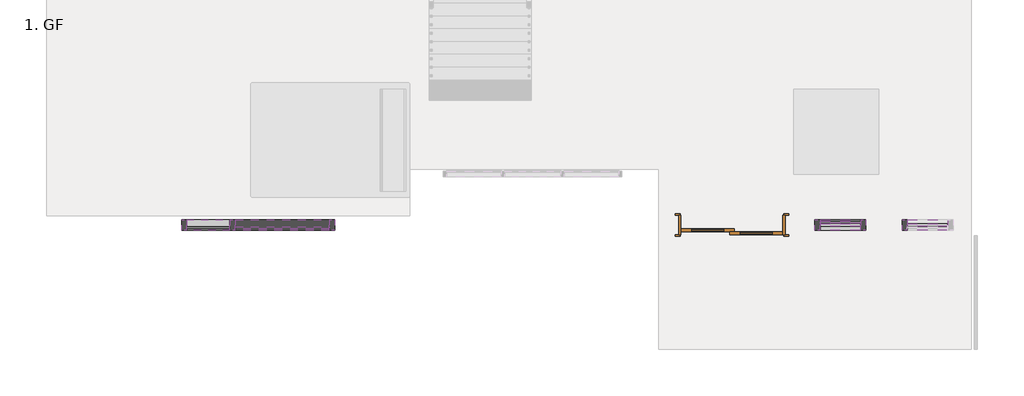
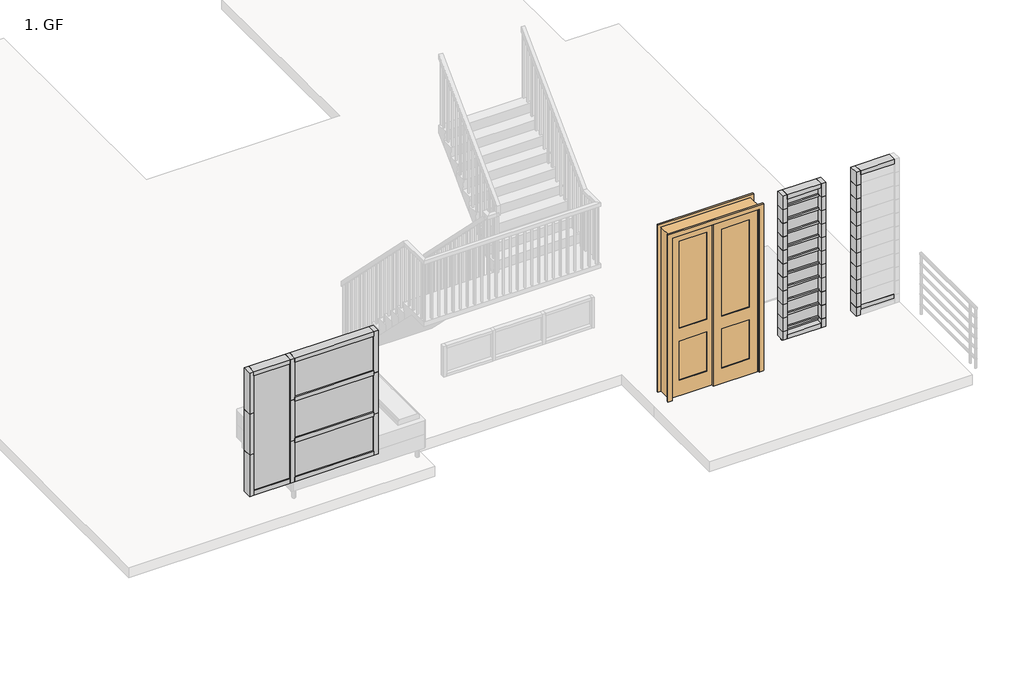
# One storey, part 1 of 3: 72 members, 16 plates, 1 door.
"""IFC4 building model written with IfcOpenShell, lengths in millimetres."""

from ifc_helpers import new_model, si_unit, origin, place, context, project, spatial, transform, mapped, element, save
from components import door_interior_double_sliding_2_panel_wood_4_x8_84ebb68c, member_93b5357b, member_3e1f1dd8, member_86d06fe4, member_a8054089, member_a8e3eee7, member_0b7646a3, member_e6b9f524, member_2cd1b1d9, member_866a01fa, member_c3a59c23, system_panel_glazed_ee894bee, system_panel_glazed_9eb8e914, system_panel_glazed_008e37cc, system_panel_glazed_06acdacc, system_panel_glazed_f6e37d5f, system_panel_glazed_d1e8daba

model = new_model("IFC4")

# Units and contexts
model_context = context("Model", 3, world=origin())
ifc_project = project(units=[si_unit("LENGTHUNIT", "METRE", prefix="MILLI")], contexts=[model_context])

# Site, building, storey
site = spatial("IfcSite", under=ifc_project)
building = spatial("IfcBuilding", under=site)
storey = spatial("IfcBuildingStorey", under=building, Name="1. GF", Elevation=609.6)

# Door
placement = place(None, origin())
door_interior_double_sliding_2_panel_wood_4_x8_shape = door_interior_double_sliding_2_panel_wood_4_x8_84ebb68c(model_context)
element("IfcDoor", 1, ObjectType="Door-Interior-Double-Sliding-2_Panel-Wood : 4' X8'", at=placement, inside=storey, context=model_context, shape_type="MappedRepresentation", body=[
    mapped(door_interior_double_sliding_2_panel_wood_4_x8_shape, transform((855.0250448, -610.2589711, 609.6), x_axis=(-1.0, 0.0, 0.0), y_axis=(0.0, -1.0, 0.0), z_axis=(0.0, 0.0, 1.0))),
])

# Members
member_shape = member_93b5357b(model_context)
element("IfcMember", 2, ObjectType="Rectangular Mullion : 1\" Square", at=placement, inside=storey, context=model_context, shape_type="MappedRepresentation", body=[
    mapped(member_shape, transform((2391.7250448, -607.0839711, 2463.8), x_axis=(0.0, 0.0, 1.0), y_axis=(0.0, -1.0, 0.0), z_axis=(1.0, 0.0, 0.0))),
])
element("IfcMember", 3, ObjectType="Rectangular Mullion : 1\" Square", at=placement, inside=storey, context=model_context, shape_type="MappedRepresentation", body=[
    mapped(member_shape, transform((2391.7250448, -607.0839711, 2667.0), x_axis=(0.0, 0.0, 1.0), y_axis=(0.0, -1.0, 0.0), z_axis=(1.0, 0.0, 0.0))),
])
element("IfcMember", 4, ObjectType="Rectangular Mullion : 1\" Square", at=placement, inside=storey, context=model_context, shape_type="MappedRepresentation", body=[
    mapped(member_shape, transform((2391.7250448, -607.0839711, 2260.6), x_axis=(0.0, 0.0, 1.0), y_axis=(0.0, -1.0, 0.0), z_axis=(1.0, 0.0, 0.0))),
])
element("IfcMember", 5, ObjectType="Rectangular Mullion : 1\" Square", at=placement, inside=storey, context=model_context, shape_type="MappedRepresentation", body=[
    mapped(member_shape, transform((2391.7250448, -607.0839711, 2057.4), x_axis=(0.0, 0.0, 1.0), y_axis=(0.0, -1.0, 0.0), z_axis=(1.0, 0.0, 0.0))),
])
element("IfcMember", 6, ObjectType="Rectangular Mullion : 1\" Square", at=placement, inside=storey, context=model_context, shape_type="MappedRepresentation", body=[
    mapped(member_shape, transform((2950.5250448, -607.0839711, 2870.2), x_axis=(0.0, 0.0, 1.0), y_axis=(0.0, 1.0, 0.0), z_axis=(-1.0, 0.0, 0.0))),
])
element("IfcMember", 7, ObjectType="Rectangular Mullion : 1\" Square", at=placement, inside=storey, context=model_context, shape_type="MappedRepresentation", body=[
    mapped(member_shape, transform((2950.5250448, -607.0839711, 2667.0), x_axis=(0.0, 0.0, 1.0), y_axis=(0.0, 1.0, 0.0), z_axis=(-1.0, 0.0, 0.0))),
])
element("IfcMember", 8, ObjectType="Rectangular Mullion : 1\" Square", at=placement, inside=storey, context=model_context, shape_type="MappedRepresentation", body=[
    mapped(member_shape, transform((2950.5250448, -607.0839711, 2463.8), x_axis=(0.0, 0.0, 1.0), y_axis=(0.0, 1.0, 0.0), z_axis=(-1.0, 0.0, 0.0))),
])
element("IfcMember", 9, ObjectType="Rectangular Mullion : 1\" Square", at=placement, inside=storey, context=model_context, shape_type="MappedRepresentation", body=[
    mapped(member_shape, transform((2950.5250448, -607.0839711, 2260.6), x_axis=(0.0, 0.0, 1.0), y_axis=(0.0, 1.0, 0.0), z_axis=(-1.0, 0.0, 0.0))),
])
element("IfcMember", 10, ObjectType="Rectangular Mullion : 1\" Square", at=placement, inside=storey, context=model_context, shape_type="MappedRepresentation", body=[
    mapped(member_shape, transform((2950.5250448, -607.0839711, 2057.4), x_axis=(0.0, 0.0, 1.0), y_axis=(0.0, 1.0, 0.0), z_axis=(-1.0, 0.0, 0.0))),
])
element("IfcMember", 11, ObjectType="Rectangular Mullion : 1\" Square", at=placement, inside=storey, context=model_context, shape_type="MappedRepresentation", body=[
    mapped(member_shape, transform((2950.5250448, -607.0839711, 1854.2), x_axis=(0.0, 0.0, 1.0), y_axis=(0.0, 1.0, 0.0), z_axis=(-1.0, 0.0, 0.0))),
])
element("IfcMember", 12, ObjectType="Rectangular Mullion : 1\" Square", at=placement, inside=storey, context=model_context, shape_type="MappedRepresentation", body=[
    mapped(member_shape, transform((2950.5250448, -607.0839711, 1651.0), x_axis=(0.0, 0.0, 1.0), y_axis=(0.0, 1.0, 0.0), z_axis=(-1.0, 0.0, 0.0))),
])
element("IfcMember", 13, ObjectType="Rectangular Mullion : 1\" Square", at=placement, inside=storey, context=model_context, shape_type="MappedRepresentation", body=[
    mapped(member_shape, transform((2950.5250448, -607.0839711, 1447.8), x_axis=(0.0, 0.0, 1.0), y_axis=(0.0, 1.0, 0.0), z_axis=(-1.0, 0.0, 0.0))),
])
element("IfcMember", 14, ObjectType="Rectangular Mullion : 1\" Square", at=placement, inside=storey, context=model_context, shape_type="MappedRepresentation", body=[
    mapped(member_shape, transform((2950.5250448, -607.0839711, 1244.6), x_axis=(0.0, 0.0, 1.0), y_axis=(0.0, 1.0, 0.0), z_axis=(-1.0, 0.0, 0.0))),
])
element("IfcMember", 15, ObjectType="Rectangular Mullion : 1\" Square", at=placement, inside=storey, context=model_context, shape_type="MappedRepresentation", body=[
    mapped(member_shape, transform((2950.5250448, -607.0839711, 1041.4), x_axis=(0.0, 0.0, 1.0), y_axis=(0.0, 1.0, 0.0), z_axis=(-1.0, 0.0, 0.0))),
])
element("IfcMember", 16, ObjectType="Rectangular Mullion : 1\" Square", at=placement, inside=storey, context=model_context, shape_type="MappedRepresentation", body=[
    mapped(member_shape, transform((2391.7250448, -607.0839711, 1447.8), x_axis=(0.0, 0.0, 1.0), y_axis=(0.0, -1.0, 0.0), z_axis=(1.0, 0.0, 0.0))),
])
element("IfcMember", 17, ObjectType="Rectangular Mullion : 1\" Square", at=placement, inside=storey, context=model_context, shape_type="MappedRepresentation", body=[
    mapped(member_shape, transform((2391.7250448, -607.0839711, 1651.0), x_axis=(0.0, 0.0, 1.0), y_axis=(0.0, -1.0, 0.0), z_axis=(1.0, 0.0, 0.0))),
])
element("IfcMember", 18, ObjectType="Rectangular Mullion : 1\" Square", at=placement, inside=storey, context=model_context, shape_type="MappedRepresentation", body=[
    mapped(member_shape, transform((2391.7250448, -607.0839711, 1854.2), x_axis=(0.0, 0.0, 1.0), y_axis=(0.0, -1.0, 0.0), z_axis=(1.0, 0.0, 0.0))),
])
element("IfcMember", 19, ObjectType="Rectangular Mullion : 1\" Square", at=placement, inside=storey, context=model_context, shape_type="MappedRepresentation", body=[
    mapped(member_shape, transform((2391.7250448, -607.0839711, 1244.6), x_axis=(0.0, 0.0, 1.0), y_axis=(0.0, -1.0, 0.0), z_axis=(1.0, 0.0, 0.0))),
])
element("IfcMember", 20, ObjectType="Rectangular Mullion : 1\" Square", at=placement, inside=storey, context=model_context, shape_type="MappedRepresentation", body=[
    mapped(member_shape, transform((2391.7250448, -607.0839711, 1041.4), x_axis=(0.0, 0.0, 1.0), y_axis=(0.0, -1.0, 0.0), z_axis=(1.0, 0.0, 0.0))),
])
element("IfcMember", 21, ObjectType="Rectangular Mullion : 1\" Square", at=placement, inside=storey, context=model_context, shape_type="MappedRepresentation", body=[
    mapped(member_shape, transform((2391.7250448, -607.0839711, 2870.2), x_axis=(0.0, 0.0, 1.0), y_axis=(0.0, -1.0, 0.0), z_axis=(1.0, 0.0, 0.0))),
])
member_2_shape = member_3e1f1dd8(model_context)
element("IfcMember", 22, ObjectType="Rectangular Mullion : 1\" Square", at=placement, inside=storey, context=model_context, shape_type="MappedRepresentation", body=[
    mapped(member_2_shape, transform((1845.6250448, -632.4839711, 914.4), x_axis=(0.0, 0.0, -1.0), y_axis=(0.0, -1.0, 0.0), z_axis=(-1.0, 0.0, 0.0))),
])
member_3_shape = member_86d06fe4(model_context)
element("IfcMember", 23, ObjectType="Rectangular Mullion : 2.5\" x 5\" rectangular", at=placement, inside=storey, context=model_context, shape_type="MappedRepresentation", body=[
    mapped(member_3_shape, transform((2391.7250448, -607.0839711, 3073.4), x_axis=(0.0, 0.0, 1.0), y_axis=(0.0, -1.0, 0.0), z_axis=(1.0, 0.0, 0.0))),
])
element("IfcMember", 24, ObjectType="Rectangular Mullion : 2.5\" x 5\" rectangular", at=placement, inside=storey, context=model_context, shape_type="MappedRepresentation", body=[
    mapped(member_3_shape, transform((2950.5250448, -607.0839711, 3073.4), x_axis=(0.0, 0.0, 1.0), y_axis=(0.0, 1.0, 0.0), z_axis=(-1.0, 0.0, 0.0))),
])
element("IfcMember", 25, ObjectType="Rectangular Mullion : 2.5\" x 5\" rectangular", at=placement, inside=storey, context=model_context, shape_type="MappedRepresentation", body=[
    mapped(member_3_shape, transform((1909.1250448, -607.0839711, 914.4), x_axis=(0.0, 0.0, -1.0), y_axis=(0.0, -1.0, 0.0), z_axis=(-1.0, 0.0, 0.0))),
])
member_4_shape = member_a8054089(model_context)
element("IfcMember", 26, ObjectType="Rectangular Mullion : 2.5\" x 5\" rectangular", at=placement, inside=storey, context=model_context, shape_type="MappedRepresentation", body=[
    mapped(member_4_shape, transform((1845.6250448, -607.0839711, 3073.4), x_axis=(-1.0, 0.0, 0.0), y_axis=(0.0, -1.0, 0.0), z_axis=(0.0, 0.0, 1.0))),
])
member_5_shape = member_a8e3eee7(model_context)
element("IfcMember", 27, ObjectType="Rectangular Mullion : 2.5\" x 5\" rectangular", at=placement, inside=storey, context=model_context, shape_type="MappedRepresentation", body=[
    mapped(member_5_shape, transform((2455.2250448, -607.0839711, 914.4), x_axis=(1.0, 0.0, 0.0), y_axis=(0.0, -1.0, 0.0), z_axis=(0.0, 0.0, -1.0))),
])
element("IfcMember", 28, ObjectType="Rectangular Mullion : 2.5\" x 5\" rectangular", at=placement, inside=storey, context=model_context, shape_type="MappedRepresentation", body=[
    mapped(member_5_shape, transform((2887.0250448, -607.0839711, 914.4), x_axis=(-1.0, 0.0, 0.0), y_axis=(0.0, 1.0, 0.0), z_axis=(0.0, 0.0, -1.0))),
])
element("IfcMember", 29, ObjectType="Rectangular Mullion : 2.5\" x 5\" rectangular", at=placement, inside=storey, context=model_context, shape_type="MappedRepresentation", body=[
    mapped(member_4_shape, transform((2887.0250448, -607.0839711, 2870.2), x_axis=(-1.0, 0.0, 0.0), y_axis=(0.0, 1.0, 0.0), z_axis=(0.0, 0.0, -1.0))),
])
element("IfcMember", 30, ObjectType="Rectangular Mullion : 2.5\" x 5\" rectangular", at=placement, inside=storey, context=model_context, shape_type="MappedRepresentation", body=[
    mapped(member_4_shape, transform((2455.2250448, -607.0839711, 2870.2), x_axis=(1.0, 0.0, 0.0), y_axis=(0.0, -1.0, 0.0), z_axis=(0.0, 0.0, -1.0))),
])
element("IfcMember", 31, ObjectType="Rectangular Mullion : 2.5\" x 5\" rectangular", at=placement, inside=storey, context=model_context, shape_type="MappedRepresentation", body=[
    mapped(member_4_shape, transform((2455.2250448, -607.0839711, 2667.0), x_axis=(1.0, 0.0, 0.0), y_axis=(0.0, -1.0, 0.0), z_axis=(0.0, 0.0, -1.0))),
])
element("IfcMember", 32, ObjectType="Rectangular Mullion : 2.5\" x 5\" rectangular", at=placement, inside=storey, context=model_context, shape_type="MappedRepresentation", body=[
    mapped(member_4_shape, transform((2455.2250448, -607.0839711, 2463.8), x_axis=(1.0, 0.0, 0.0), y_axis=(0.0, -1.0, 0.0), z_axis=(0.0, 0.0, -1.0))),
])
element("IfcMember", 33, ObjectType="Rectangular Mullion : 2.5\" x 5\" rectangular", at=placement, inside=storey, context=model_context, shape_type="MappedRepresentation", body=[
    mapped(member_4_shape, transform((2455.2250448, -607.0839711, 2260.6), x_axis=(1.0, 0.0, 0.0), y_axis=(0.0, -1.0, 0.0), z_axis=(0.0, 0.0, -1.0))),
])
element("IfcMember", 34, ObjectType="Rectangular Mullion : 2.5\" x 5\" rectangular", at=placement, inside=storey, context=model_context, shape_type="MappedRepresentation", body=[
    mapped(member_4_shape, transform((2455.2250448, -607.0839711, 2057.4), x_axis=(1.0, 0.0, 0.0), y_axis=(0.0, -1.0, 0.0), z_axis=(0.0, 0.0, -1.0))),
])
element("IfcMember", 35, ObjectType="Rectangular Mullion : 2.5\" x 5\" rectangular", at=placement, inside=storey, context=model_context, shape_type="MappedRepresentation", body=[
    mapped(member_4_shape, transform((2455.2250448, -607.0839711, 1854.2), x_axis=(1.0, 0.0, 0.0), y_axis=(0.0, -1.0, 0.0), z_axis=(0.0, 0.0, -1.0))),
])
element("IfcMember", 36, ObjectType="Rectangular Mullion : 2.5\" x 5\" rectangular", at=placement, inside=storey, context=model_context, shape_type="MappedRepresentation", body=[
    mapped(member_4_shape, transform((2455.2250448, -607.0839711, 1651.0), x_axis=(1.0, 0.0, 0.0), y_axis=(0.0, -1.0, 0.0), z_axis=(0.0, 0.0, -1.0))),
])
element("IfcMember", 37, ObjectType="Rectangular Mullion : 2.5\" x 5\" rectangular", at=placement, inside=storey, context=model_context, shape_type="MappedRepresentation", body=[
    mapped(member_4_shape, transform((2455.2250448, -607.0839711, 1447.8), x_axis=(1.0, 0.0, 0.0), y_axis=(0.0, -1.0, 0.0), z_axis=(0.0, 0.0, -1.0))),
])
element("IfcMember", 38, ObjectType="Rectangular Mullion : 2.5\" x 5\" rectangular", at=placement, inside=storey, context=model_context, shape_type="MappedRepresentation", body=[
    mapped(member_4_shape, transform((2455.2250448, -607.0839711, 1244.6), x_axis=(1.0, 0.0, 0.0), y_axis=(0.0, -1.0, 0.0), z_axis=(0.0, 0.0, -1.0))),
])
element("IfcMember", 39, ObjectType="Rectangular Mullion : 2.5\" x 5\" rectangular", at=placement, inside=storey, context=model_context, shape_type="MappedRepresentation", body=[
    mapped(member_4_shape, transform((2455.2250448, -607.0839711, 1041.4), x_axis=(1.0, 0.0, 0.0), y_axis=(0.0, -1.0, 0.0), z_axis=(0.0, 0.0, -1.0))),
])
element("IfcMember", 40, ObjectType="Rectangular Mullion : 2.5\" x 5\" rectangular", at=placement, inside=storey, context=model_context, shape_type="MappedRepresentation", body=[
    mapped(member_4_shape, transform((2887.0250448, -607.0839711, 2667.0), x_axis=(-1.0, 0.0, 0.0), y_axis=(0.0, 1.0, 0.0), z_axis=(0.0, 0.0, -1.0))),
])
element("IfcMember", 41, ObjectType="Rectangular Mullion : 2.5\" x 5\" rectangular", at=placement, inside=storey, context=model_context, shape_type="MappedRepresentation", body=[
    mapped(member_4_shape, transform((2887.0250448, -607.0839711, 2463.8), x_axis=(-1.0, 0.0, 0.0), y_axis=(0.0, 1.0, 0.0), z_axis=(0.0, 0.0, -1.0))),
])
element("IfcMember", 42, ObjectType="Rectangular Mullion : 2.5\" x 5\" rectangular", at=placement, inside=storey, context=model_context, shape_type="MappedRepresentation", body=[
    mapped(member_4_shape, transform((2887.0250448, -607.0839711, 2260.6), x_axis=(-1.0, 0.0, 0.0), y_axis=(0.0, 1.0, 0.0), z_axis=(0.0, 0.0, -1.0))),
])
element("IfcMember", 43, ObjectType="Rectangular Mullion : 2.5\" x 5\" rectangular", at=placement, inside=storey, context=model_context, shape_type="MappedRepresentation", body=[
    mapped(member_4_shape, transform((2887.0250448, -607.0839711, 2057.4), x_axis=(-1.0, 0.0, 0.0), y_axis=(0.0, 1.0, 0.0), z_axis=(0.0, 0.0, -1.0))),
])
element("IfcMember", 44, ObjectType="Rectangular Mullion : 2.5\" x 5\" rectangular", at=placement, inside=storey, context=model_context, shape_type="MappedRepresentation", body=[
    mapped(member_4_shape, transform((2887.0250448, -607.0839711, 1854.2), x_axis=(-1.0, 0.0, 0.0), y_axis=(0.0, 1.0, 0.0), z_axis=(0.0, 0.0, -1.0))),
])
element("IfcMember", 45, ObjectType="Rectangular Mullion : 2.5\" x 5\" rectangular", at=placement, inside=storey, context=model_context, shape_type="MappedRepresentation", body=[
    mapped(member_4_shape, transform((2887.0250448, -607.0839711, 1651.0), x_axis=(-1.0, 0.0, 0.0), y_axis=(0.0, 1.0, 0.0), z_axis=(0.0, 0.0, -1.0))),
])
element("IfcMember", 46, ObjectType="Rectangular Mullion : 2.5\" x 5\" rectangular", at=placement, inside=storey, context=model_context, shape_type="MappedRepresentation", body=[
    mapped(member_4_shape, transform((2887.0250448, -607.0839711, 1447.8), x_axis=(-1.0, 0.0, 0.0), y_axis=(0.0, 1.0, 0.0), z_axis=(0.0, 0.0, -1.0))),
])
element("IfcMember", 47, ObjectType="Rectangular Mullion : 2.5\" x 5\" rectangular", at=placement, inside=storey, context=model_context, shape_type="MappedRepresentation", body=[
    mapped(member_4_shape, transform((2887.0250448, -607.0839711, 1244.6), x_axis=(-1.0, 0.0, 0.0), y_axis=(0.0, 1.0, 0.0), z_axis=(0.0, 0.0, -1.0))),
])
element("IfcMember", 48, ObjectType="Rectangular Mullion : 2.5\" x 5\" rectangular", at=placement, inside=storey, context=model_context, shape_type="MappedRepresentation", body=[
    mapped(member_4_shape, transform((2887.0250448, -607.0839711, 1041.4), x_axis=(-1.0, 0.0, 0.0), y_axis=(0.0, 1.0, 0.0), z_axis=(0.0, 0.0, -1.0))),
])
element("IfcMember", 49, ObjectType="Rectangular Mullion : 2.5\" x 5\" rectangular", at=placement, inside=storey, context=model_context, shape_type="MappedRepresentation", body=[
    mapped(member_4_shape, transform((1845.6250448, -607.0839711, 2667.0), x_axis=(-1.0, 0.0, 0.0), y_axis=(0.0, -1.0, 0.0), z_axis=(0.0, 0.0, 1.0))),
])
element("IfcMember", 50, ObjectType="Rectangular Mullion : 2.5\" x 5\" rectangular", at=placement, inside=storey, context=model_context, shape_type="MappedRepresentation", body=[
    mapped(member_4_shape, transform((1845.6250448, -607.0839711, 2463.8), x_axis=(-1.0, 0.0, 0.0), y_axis=(0.0, -1.0, 0.0), z_axis=(0.0, 0.0, 1.0))),
])
element("IfcMember", 51, ObjectType="Rectangular Mullion : 2.5\" x 5\" rectangular", at=placement, inside=storey, context=model_context, shape_type="MappedRepresentation", body=[
    mapped(member_4_shape, transform((1845.6250448, -607.0839711, 2260.6), x_axis=(-1.0, 0.0, 0.0), y_axis=(0.0, -1.0, 0.0), z_axis=(0.0, 0.0, 1.0))),
])
element("IfcMember", 52, ObjectType="Rectangular Mullion : 2.5\" x 5\" rectangular", at=placement, inside=storey, context=model_context, shape_type="MappedRepresentation", body=[
    mapped(member_4_shape, transform((1845.6250448, -607.0839711, 2057.4), x_axis=(-1.0, 0.0, 0.0), y_axis=(0.0, -1.0, 0.0), z_axis=(0.0, 0.0, 1.0))),
])
element("IfcMember", 53, ObjectType="Rectangular Mullion : 2.5\" x 5\" rectangular", at=placement, inside=storey, context=model_context, shape_type="MappedRepresentation", body=[
    mapped(member_4_shape, transform((1845.6250448, -607.0839711, 1854.2), x_axis=(-1.0, 0.0, 0.0), y_axis=(0.0, -1.0, 0.0), z_axis=(0.0, 0.0, 1.0))),
])
element("IfcMember", 54, ObjectType="Rectangular Mullion : 2.5\" x 5\" rectangular", at=placement, inside=storey, context=model_context, shape_type="MappedRepresentation", body=[
    mapped(member_4_shape, transform((1845.6250448, -607.0839711, 1651.0), x_axis=(-1.0, 0.0, 0.0), y_axis=(0.0, -1.0, 0.0), z_axis=(0.0, 0.0, 1.0))),
])
element("IfcMember", 55, ObjectType="Rectangular Mullion : 2.5\" x 5\" rectangular", at=placement, inside=storey, context=model_context, shape_type="MappedRepresentation", body=[
    mapped(member_4_shape, transform((1845.6250448, -607.0839711, 1447.8), x_axis=(-1.0, 0.0, 0.0), y_axis=(0.0, -1.0, 0.0), z_axis=(0.0, 0.0, 1.0))),
])
element("IfcMember", 56, ObjectType="Rectangular Mullion : 2.5\" x 5\" rectangular", at=placement, inside=storey, context=model_context, shape_type="MappedRepresentation", body=[
    mapped(member_4_shape, transform((1845.6250448, -607.0839711, 1244.6), x_axis=(-1.0, 0.0, 0.0), y_axis=(0.0, -1.0, 0.0), z_axis=(0.0, 0.0, 1.0))),
])
element("IfcMember", 57, ObjectType="Rectangular Mullion : 2.5\" x 5\" rectangular", at=placement, inside=storey, context=model_context, shape_type="MappedRepresentation", body=[
    mapped(member_4_shape, transform((1845.6250448, -607.0839711, 2870.2), x_axis=(-1.0, 0.0, 0.0), y_axis=(0.0, -1.0, 0.0), z_axis=(0.0, 0.0, 1.0))),
])
element("IfcMember", 58, ObjectType="Rectangular Mullion : 2.5\" x 5\" rectangular", at=placement, inside=storey, context=model_context, shape_type="MappedRepresentation", body=[
    mapped(member_5_shape, transform((1845.6250448, -607.0839711, 1041.4), x_axis=(-1.0, 0.0, 0.0), y_axis=(0.0, -1.0, 0.0), z_axis=(0.0, 0.0, 1.0))),
])
member_6_shape = member_0b7646a3(model_context)
element("IfcMember", 59, ObjectType="Rectangular Mullion : 2.5\" x 5\" rectangular", at=placement, inside=storey, context=model_context, shape_type="MappedRepresentation", body=[
    mapped(member_6_shape, transform((-5660.0749552, -607.0839711, 3073.4), x_axis=(0.0, 0.0, 1.0), y_axis=(0.0, 1.0, 0.0), z_axis=(-1.0, 0.0, 0.0))),
])
member_7_shape = member_e6b9f524(model_context)
element("IfcMember", 60, ObjectType="Rectangular Mullion : 2.5\" x 5\" rectangular", at=placement, inside=storey, context=model_context, shape_type="MappedRepresentation", body=[
    mapped(member_7_shape, transform((-3958.2749552, -607.0839711, 1219.2), x_axis=(0.0, 0.0, -1.0), y_axis=(0.0, 1.0, 0.0), z_axis=(1.0, 0.0, 0.0))),
])
member_8_shape = member_2cd1b1d9(model_context)
element("IfcMember", 61, ObjectType="Rectangular Mullion : 2.5\" x 5\" rectangular", at=placement, inside=storey, context=model_context, shape_type="MappedRepresentation", body=[
    mapped(member_8_shape, transform((-5113.9749552, -607.0839711, 1219.2), x_axis=(-1.0, 0.0, 0.0), y_axis=(0.0, 1.0, 0.0), z_axis=(0.0, 0.0, -1.0))),
])
member_9_shape = member_866a01fa(model_context)
element("IfcMember", 62, ObjectType="Rectangular Mullion : 2.5\" x 5\" rectangular", at=placement, inside=storey, context=model_context, shape_type="MappedRepresentation", body=[
    mapped(member_9_shape, transform((-5082.2249552, -607.0839711, 2455.3333333), x_axis=(0.0, 0.0, 1.0), y_axis=(0.0, 1.0, 0.0), z_axis=(-1.0, 0.0, 0.0))),
])
element("IfcMember", 63, ObjectType="Rectangular Mullion : 2.5\" x 5\" rectangular", at=placement, inside=storey, context=model_context, shape_type="MappedRepresentation", body=[
    mapped(member_9_shape, transform((-5082.2249552, -607.0839711, 1837.2666667), x_axis=(0.0, 0.0, 1.0), y_axis=(0.0, 1.0, 0.0), z_axis=(-1.0, 0.0, 0.0))),
])
element("IfcMember", 64, ObjectType="Rectangular Mullion : 2.5\" x 5\" rectangular", at=placement, inside=storey, context=model_context, shape_type="MappedRepresentation", body=[
    mapped(member_6_shape, transform((-5145.7249552, -607.0839711, 1219.2), x_axis=(0.0, 0.0, -1.0), y_axis=(0.0, 1.0, 0.0), z_axis=(1.0, 0.0, 0.0))),
])
element("IfcMember", 65, ObjectType="Rectangular Mullion : 2.5\" x 5\" rectangular", at=placement, inside=storey, context=model_context, shape_type="MappedRepresentation", body=[
    mapped(member_7_shape, transform((-5082.2249552, -607.0839711, 3073.4), x_axis=(0.0, 0.0, 1.0), y_axis=(0.0, 1.0, 0.0), z_axis=(-1.0, 0.0, 0.0))),
])
element("IfcMember", 66, ObjectType="Rectangular Mullion : 2.5\" x 5\" rectangular", at=placement, inside=storey, context=model_context, shape_type="MappedRepresentation", body=[
    mapped(member_8_shape, transform((-5113.9749552, -607.0839711, 2455.3333333), x_axis=(-1.0, 0.0, 0.0), y_axis=(0.0, 1.0, 0.0), z_axis=(0.0, 0.0, -1.0))),
])
element("IfcMember", 67, ObjectType="Rectangular Mullion : 2.5\" x 5\" rectangular", at=placement, inside=storey, context=model_context, shape_type="MappedRepresentation", body=[
    mapped(member_8_shape, transform((-5113.9749552, -607.0839711, 1837.2666667), x_axis=(-1.0, 0.0, 0.0), y_axis=(0.0, 1.0, 0.0), z_axis=(0.0, 0.0, -1.0))),
])
member_10_shape = member_c3a59c23(model_context)
element("IfcMember", 68, ObjectType="Rectangular Mullion : 2.5\" x 5\" rectangular", at=placement, inside=storey, context=model_context, shape_type="MappedRepresentation", body=[
    mapped(member_10_shape, transform((-3894.7749552, -607.0839711, 3073.4), x_axis=(1.0, 0.0, 0.0), y_axis=(0.0, 1.0, 0.0), z_axis=(0.0, 0.0, 1.0))),
])
element("IfcMember", 69, ObjectType="Rectangular Mullion : 2.5\" x 5\" rectangular", at=placement, inside=storey, context=model_context, shape_type="MappedRepresentation", body=[
    mapped(member_10_shape, transform((-5723.5749552, -607.0839711, 1219.2), x_axis=(-1.0, 0.0, 0.0), y_axis=(0.0, 1.0, 0.0), z_axis=(0.0, 0.0, -1.0))),
])
element("IfcMember", 70, ObjectType="Rectangular Mullion : 2.5\" x 5\" rectangular", at=placement, inside=storey, context=model_context, shape_type="MappedRepresentation", body=[
    mapped(member_10_shape, transform((-5723.5749552, -607.0839711, 2455.3333333), x_axis=(-1.0, 0.0, 0.0), y_axis=(0.0, 1.0, 0.0), z_axis=(0.0, 0.0, -1.0))),
])
element("IfcMember", 71, ObjectType="Rectangular Mullion : 2.5\" x 5\" rectangular", at=placement, inside=storey, context=model_context, shape_type="MappedRepresentation", body=[
    mapped(member_10_shape, transform((-5723.5749552, -607.0839711, 1837.2666667), x_axis=(-1.0, 0.0, 0.0), y_axis=(0.0, 1.0, 0.0), z_axis=(0.0, 0.0, -1.0))),
])
element("IfcMember", 72, ObjectType="Rectangular Mullion : 2.5\" x 5\" rectangular", at=placement, inside=storey, context=model_context, shape_type="MappedRepresentation", body=[
    mapped(member_10_shape, transform((-3894.7749552, -607.0839711, 2455.3333333), x_axis=(1.0, 0.0, 0.0), y_axis=(0.0, 1.0, 0.0), z_axis=(0.0, 0.0, 1.0))),
])
element("IfcMember", 73, ObjectType="Rectangular Mullion : 2.5\" x 5\" rectangular", at=placement, inside=storey, context=model_context, shape_type="MappedRepresentation", body=[
    mapped(member_10_shape, transform((-3894.7749552, -607.0839711, 1837.2666667), x_axis=(1.0, 0.0, 0.0), y_axis=(0.0, 1.0, 0.0), z_axis=(0.0, 0.0, 1.0))),
])

# Plates
system_panel_glazed_shape = system_panel_glazed_ee894bee(model_context)
element("IfcPlate", 74, ObjectType="System Panel : Glazed", at=placement, inside=storey, context=model_context, shape_type="MappedRepresentation", body=[
    mapped(system_panel_glazed_shape, transform((2150.4250448, -607.0839711, 977.9), x_axis=(1.0, 0.0, 0.0), y_axis=(0.0, 1.0, 0.0), z_axis=(0.0, 0.0, 1.0))),
])
element("IfcPlate", 75, ObjectType="System Panel : Glazed", at=placement, inside=storey, context=model_context, shape_type="MappedRepresentation", body=[
    mapped(system_panel_glazed_shape, transform((3191.8250448, -607.0839711, 977.9), x_axis=(-1.0, 0.0, 0.0), y_axis=(0.0, -1.0, 0.0), z_axis=(0.0, 0.0, 1.0))),
])
system_panel_glazed_2_shape = system_panel_glazed_9eb8e914(model_context)
element("IfcPlate", 76, ObjectType="System Panel : Glazed", at=placement, inside=storey, context=model_context, shape_type="MappedRepresentation", body=[
    mapped(system_panel_glazed_2_shape, transform((2150.4250448, -607.0839711, 2667.0), x_axis=(1.0, 0.0, 0.0), y_axis=(0.0, 1.0, 0.0), z_axis=(0.0, 0.0, 1.0))),
])
element("IfcPlate", 77, ObjectType="System Panel : Glazed", at=placement, inside=storey, context=model_context, shape_type="MappedRepresentation", body=[
    mapped(system_panel_glazed_2_shape, transform((2150.4250448, -607.0839711, 2463.8), x_axis=(1.0, 0.0, 0.0), y_axis=(0.0, 1.0, 0.0), z_axis=(0.0, 0.0, 1.0))),
])
element("IfcPlate", 78, ObjectType="System Panel : Glazed", at=placement, inside=storey, context=model_context, shape_type="MappedRepresentation", body=[
    mapped(system_panel_glazed_2_shape, transform((2150.4250448, -607.0839711, 2260.6), x_axis=(1.0, 0.0, 0.0), y_axis=(0.0, 1.0, 0.0), z_axis=(0.0, 0.0, 1.0))),
])
element("IfcPlate", 79, ObjectType="System Panel : Glazed", at=placement, inside=storey, context=model_context, shape_type="MappedRepresentation", body=[
    mapped(system_panel_glazed_2_shape, transform((2150.4250448, -607.0839711, 2057.4), x_axis=(1.0, 0.0, 0.0), y_axis=(0.0, 1.0, 0.0), z_axis=(0.0, 0.0, 1.0))),
])
element("IfcPlate", 80, ObjectType="System Panel : Glazed", at=placement, inside=storey, context=model_context, shape_type="MappedRepresentation", body=[
    mapped(system_panel_glazed_2_shape, transform((2150.4250448, -607.0839711, 1854.2), x_axis=(1.0, 0.0, 0.0), y_axis=(0.0, 1.0, 0.0), z_axis=(0.0, 0.0, 1.0))),
])
element("IfcPlate", 81, ObjectType="System Panel : Glazed", at=placement, inside=storey, context=model_context, shape_type="MappedRepresentation", body=[
    mapped(system_panel_glazed_2_shape, transform((2150.4250448, -607.0839711, 1651.0), x_axis=(1.0, 0.0, 0.0), y_axis=(0.0, 1.0, 0.0), z_axis=(0.0, 0.0, 1.0))),
])
element("IfcPlate", 82, ObjectType="System Panel : Glazed", at=placement, inside=storey, context=model_context, shape_type="MappedRepresentation", body=[
    mapped(system_panel_glazed_2_shape, transform((2150.4250448, -607.0839711, 1447.8), x_axis=(1.0, 0.0, 0.0), y_axis=(0.0, 1.0, 0.0), z_axis=(0.0, 0.0, 1.0))),
])
element("IfcPlate", 83, ObjectType="System Panel : Glazed", at=placement, inside=storey, context=model_context, shape_type="MappedRepresentation", body=[
    mapped(system_panel_glazed_2_shape, transform((2150.4250448, -607.0839711, 1244.6), x_axis=(1.0, 0.0, 0.0), y_axis=(0.0, 1.0, 0.0), z_axis=(0.0, 0.0, 1.0))),
])
element("IfcPlate", 84, ObjectType="System Panel : Glazed", at=placement, inside=storey, context=model_context, shape_type="MappedRepresentation", body=[
    mapped(system_panel_glazed_2_shape, transform((2150.4250448, -607.0839711, 1041.4), x_axis=(1.0, 0.0, 0.0), y_axis=(0.0, 1.0, 0.0), z_axis=(0.0, 0.0, 1.0))),
])
system_panel_glazed_3_shape = system_panel_glazed_008e37cc(model_context)
element("IfcPlate", 85, ObjectType="System Panel : Glazed", at=placement, inside=storey, context=model_context, shape_type="MappedRepresentation", body=[
    mapped(system_panel_glazed_3_shape, transform((2150.4250448, -607.0839711, 2870.2), x_axis=(1.0, 0.0, 0.0), y_axis=(0.0, 1.0, 0.0), z_axis=(0.0, 0.0, 1.0))),
])
system_panel_glazed_4_shape = system_panel_glazed_06acdacc(model_context)
element("IfcPlate", 86, ObjectType="System Panel : Glazed", at=placement, inside=storey, context=model_context, shape_type="MappedRepresentation", body=[
    mapped(system_panel_glazed_4_shape, transform((-4520.2499552, -607.0839711, 1282.7), x_axis=(-1.0, 0.0, 0.0), y_axis=(0.0, -1.0, 0.0), z_axis=(0.0, 0.0, 1.0))),
])
element("IfcPlate", 87, ObjectType="System Panel : Glazed", at=placement, inside=storey, context=model_context, shape_type="MappedRepresentation", body=[
    mapped(system_panel_glazed_4_shape, transform((-4520.2499552, -607.0839711, 2487.0833333), x_axis=(-1.0, 0.0, 0.0), y_axis=(0.0, -1.0, 0.0), z_axis=(0.0, 0.0, 1.0))),
])
system_panel_glazed_5_shape = system_panel_glazed_f6e37d5f(model_context)
element("IfcPlate", 88, ObjectType="System Panel : Glazed", at=placement, inside=storey, context=model_context, shape_type="MappedRepresentation", body=[
    mapped(system_panel_glazed_5_shape, transform((-5402.8999552, -607.0839711, 1282.7), x_axis=(-1.0, 0.0, 0.0), y_axis=(0.0, -1.0, 0.0), z_axis=(0.0, 0.0, 1.0))),
])
system_panel_glazed_6_shape = system_panel_glazed_d1e8daba(model_context)
element("IfcPlate", 89, ObjectType="System Panel : Glazed", at=placement, inside=storey, context=model_context, shape_type="MappedRepresentation", body=[
    mapped(system_panel_glazed_6_shape, transform((-4520.2499552, -607.0839711, 1869.0166667), x_axis=(-1.0, 0.0, 0.0), y_axis=(0.0, -1.0, 0.0), z_axis=(0.0, 0.0, 1.0))),
])

save(model, "model.ifc")

# Revit data of these elements
# Type "Door-Interior-Double-Sliding-2_Panel-Wood : 4' X8'"
#   Type Mark = "13"
#   Assembly Code = "C1020300"
#   Analytic Construction = "Wooden"
#   Top Rail = 0' - 4 11/16"
#   Thickness = 0' - 1 3/8"
#   Thermal Resistance (R) = 2.5876 (h·ft²·°F)/BTU
#   Stiles = 0' - 4 3/4"
#   Rough Width = 4' - 2"
#   Rough Height = 8' - 1"
#   Lock Rail = 0' - 7 1/2"
#   Height = 8' - 0"
#   Width = 4' - 0"
#   Heat Transfer Coefficient (U) = 0.3865 BTU/(h·ft²·°F)
#   Bottom Rail = 0' - 9 1/8"
#   Trim Material = Cherry
#   Panel Material = Cherry
#   Frame Material = Cherry
#   Visual Light Transmittance = 0
#   Solar Heat Gain Coefficient = 0
#   Wall Closure = (empty or 0)
#   Function = (empty or 0)
# Type "Rectangular Mullion : 1\" Square"
#   built-in parameter 1007304 = 0.0833333 (stored number, unit not read)
#   built-in parameter 1007301 = 0.0416667 (stored number, unit not read)
#   built-in parameter 1007300 = 0.0416667 (stored number, unit not read)
# Type "Rectangular Mullion : 2.5\" x 5\" rectangular"
#   built-in parameter 1007304 = 0.416667 (stored number, unit not read)
#   built-in parameter 1007301 = 0.104167 (stored number, unit not read)
#   built-in parameter 1007300 = 0.104167 (stored number, unit not read)
# Type "System Panel : Glazed"
#   Construction Type Id = "GSP4R"
#   Analytic Construction = "1/8 in Pilkington single glazing"
#   Visual Light Transmittance = 0.9
#   Solar Heat Gain Coefficient = 0.86
#   Heat Transfer Coefficient (U) = 1.18115 BTU/(h·ft²·°F)
#   Define Thermal Properties by = 1
# Element 1 (IfcDoor, "Door-Interior-Double-Sliding-2_Panel-Wood : 4' X8'")
#   Phase Created = New Construction
#   Materials on its faces: "Cherry"
# Elements 2, 3, 4, 5, 6, 7, 8, 9, 10, 11, 12, 13, 14, 15, 16, 17, 18, 19, 20, 21, 22 (IfcMember, "Rectangular Mullion : 1\" Square")
#   Phase Created = New Construction
#   Materials on its faces: "Aluminum"
# Elements 23, 24, 25, 26, 27, 28, 29, 30, 31, 32, 33, 34, 35, 36, 37, 38, 39, 40, 41, 42, 43, 44, 45, 46, 47, 48, 49, 50, 51, 52, 53, 54, 55, 56, 57, 58, 59, 60, 61, 62, 63, 64, 65, 66, 67, 68, 69, 70, 71, 72, 73 (IfcMember, "Rectangular Mullion : 2.5\" x 5\" rectangular")
#   Phase Created = New Construction
#   Materials on its faces: "Door - Frame"
# Elements 74, 75, 76, 77, 78, 79, 80, 81, 82, 83, 84, 85, 86, 87, 88, 89 (IfcPlate, "System Panel : Glazed")
#   Phase Created = New Construction
#   Materials on its faces: "Glass"
# Materials
#   "Cherry": class "Wood", colour RGB 226 177 128, transparency 0, Description = "Prunus Serotina", Cost = 0
#   "Aluminum": class "Metal", colour RGB 247 247 247, transparency 0, Description = "Aluminum 6061", Cost = 0
#   "Door - Frame": colour RGB 118 70 51, transparency 0, Cost = 0
#   "Glass": class "Glass", colour RGB 0 128 192, transparency 0.75, Description = "Soda Lime Glass", Cost = 0
